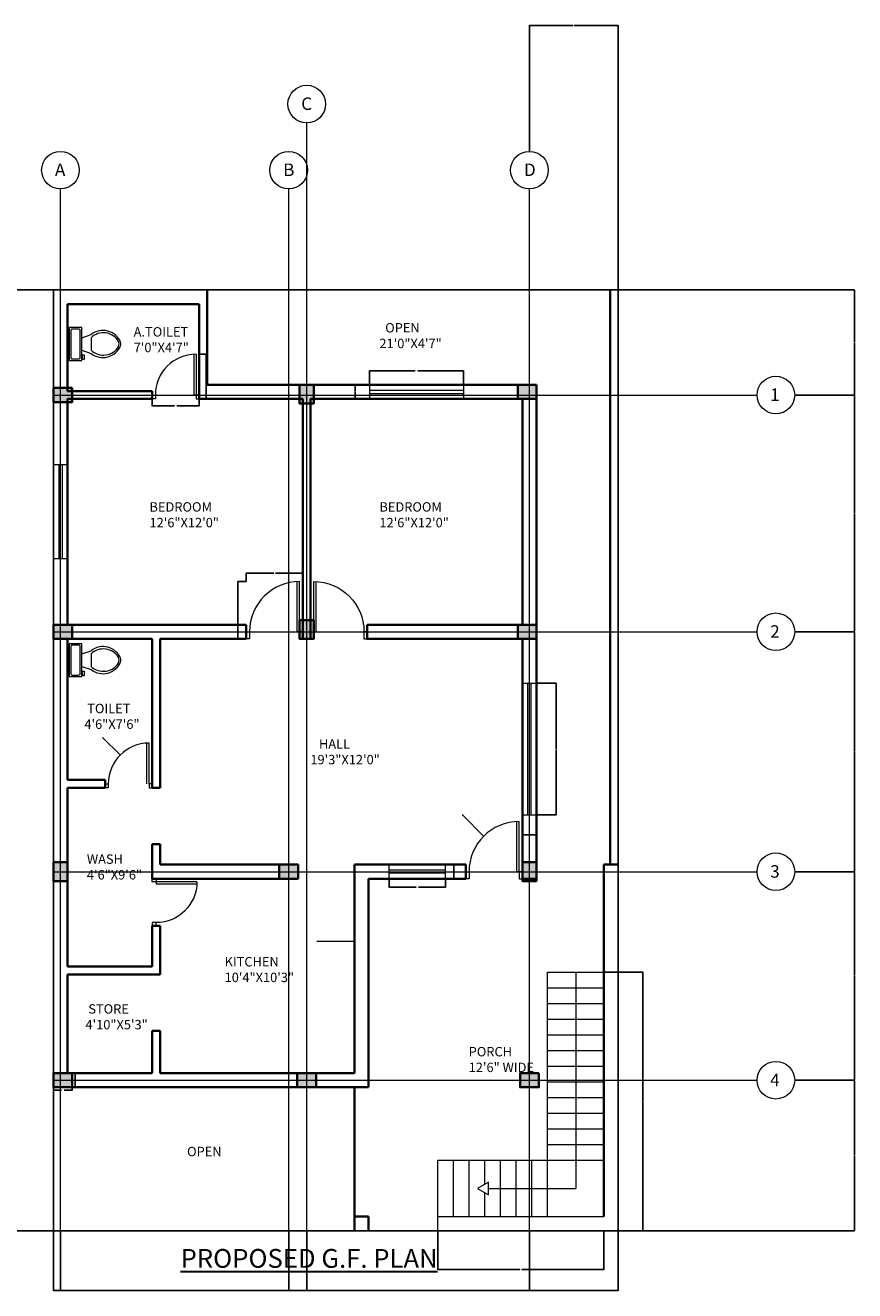
# Model space of a CAD drawing. Units: inches. Extents: x 1602 to 2642, y 1463 to 2270.
# Tile 5 of 5: x 2113 to 2642, y 1463 to 2270. Entities that reach past the tile are written whole.
import ezdxf

# ---------------------------------------------------------------- set-up
doc = ezdxf.new("R2010")
doc.units = ezdxf.units.IN
for name, color, linetype, lineweight in [('A-ANNO-DIMS', 2, 'Continuous', 18), ('A-ANNO-TEXT', 7, 'Continuous', 30), ('A-AREA-IDEN', 7, 'Continuous', 18), ('A-COLS', 7, 'Continuous', 35), ('A-DOOR', 3, 'Continuous', 18), ('A-FLOR-CASE', 9, 'Continuous', 18), ('A-FLOR-FIXT', 8, 'Continuous', 18), ('A-FLOR-STRS', 7, 'Continuous', 18), ('A-GLAZ', 4, 'Continuous', 18), ('A-GRID', 8, 'Continuous', 13), ('A-WALL', 7, 'Continuous', 35), ('C-PROP', 7, 'Continuous', 25)]:
    doc.layers.add(name, color=color, linetype=linetype, lineweight=lineweight)
doc.styles.get("Standard").update_dxf_attribs({"font": 'arial.ttf'})
doc.dimstyles.get("Standard").update_dxf_attribs({"dimtxt": 0.18, "dimasz": 0.18, "dimexe": 0.18, "dimexo": 0.0625, "dimgap": 0.09, "dimtad": 0, "dimtih": 1, "dimtoh": 1, "dimdec": 4, "dimzin": 0, "dimdsep": 46, "dimtxsty": 'Standard', "dimcen": 0.09, "dimadec": 0, "dimazin": 0, "dimtfac": 1, "dimtdec": 4, "dimtofl": 0, "dimtmove": 0, "dimatfit": 3, "dimfxl": 1, "dimtolj": 1, "dimtzin": 0, "dimarcsym": 0})

# ---------------------------------------------------------------- blocks, each defined once
blk = doc.blocks.new('*U3')
for p, q in [((-8, -8.5), (-8, -8)), ((-7, -8), (-7, -9.5)), ((-4, -8), (-6, -14)), ((4, -8), (6, -14)), ((9.5, -6), (9.5, -2)), ((-10, -8.5), (-8, -8.5)), ((-10, -9.5), (-10, -8.5)), ((-7, -9.5), (-10, -9.5)), ((4, -14), (-4, -14))]:
    blk.add_line(p, q)
blk.add_lwpolyline([(10.5, -8), (10.5, 0), (-10.5, 0), (-10.5, -8)], close=True)
for points in [[(-9.5, -2), (-9.5, -6)], [(8.5, -1), (-8.5, -1)], [(-8.5, -7), (8.5, -7)]]:
    blk.add_lwpolyline(points)
for centre, radius, start, end in [((-8.62, -1.88), 0.884, 81.8699, 188.1301), ((-8.62, -6.12), 0.884, 171.8699, 278.1301), ((8.62, -1.88), 0.884, 351.8699, 98.1301), ((8.62, -6.12), 0.884, 261.8699, 8.1301), ((3.52, -21.58), 12.17, 141.46911, 247.97143), ((4.2, -21.82), 11.33, 136.36773, 238.94682), ((-3.52, -21.58), 12.17, 292.02843, 38.53071), ((-4.2, -21.82), 11.33, 301.05301, 43.63209), ((0, -27.88), 4, 245.73182, 294.26817), ((0, -29), 4, 254.86053, 285.13947)]:
    blk.add_arc(centre, radius, start, end)
blk = doc.blocks.new('DOOR-SWING-26IN')
for p, q in [((26.5, 28.46), (26.5, 2.5)), ((28, 28.5), (28, 2.5)), ((0, 2.5), (2, 2.5)), ((2, 2.5), (2, 0)), ((28, 2.5), (26.5, 2.5)), ((30, 2.5), (28, 2.5)), ((28, 2.5), (28, 0)), ((2, 0), (0, 0)), ((28, 0), (30, 0))]:
    blk.add_line(p, q)
blk.add_arc((28, 2.5), 26, 90, 180)
blk = doc.blocks.new('DOOR-SWING-32IN')
for p, q in [((32.5, 4.5), (32.5, 36.46)), ((34, 4.5), (34, 36.5)), ((0, 4.5), (2, 4.5)), ((2, 0), (0, 0)), ((2, 4.5), (2, 0)), ((34, 4.5), (32.5, 4.5)), ((36, 4.5), (34, 4.5)), ((34, 4.5), (34, 0)), ((34, 0), (36, 0))]:
    blk.add_line(p, q)
blk.add_arc((34, 4.5), 32, 90, 180)
blk = doc.blocks.new('WIN-60IN')
for p, q in [((0, 0), (0, 9)), ((60, 0), (60, 9)), ((60, 5.5), (0, 5.5)), ((60, 3.5), (0, 3.5))]:
    blk.add_line(p, q)
blk = doc.blocks.new('WIN-36IN')
for p, q in [((0, 0), (0, 9)), ((36, 0), (36, 9)), ((36, 5.5), (0, 5.5)), ((36, 3.5), (0, 3.5))]:
    blk.add_line(p, q)
blk = doc.blocks.new('WIN-84IN')
for p, q in [((0, 84), (9, 84)), ((3.5, 0), (3.5, 84)), ((5.5, 0), (5.5, 84)), ((0, 0), (9, 0))]:
    blk.add_line(p, q)
blk = doc.blocks.new('COL-12X9')
h = blk.add_hatch(color=256)
h.dxf.hatch_style = 1
h.paths.add_polyline_path([(12, 0), (12, 9), (0, 9), (0, 0)])
blk.add_lwpolyline([(12, 9), (12, 0), (0, 0), (0, 9)], close=True)
blk = doc.blocks.new('STAIR-PORCH-RETURN')
for p, q in [((70, 9), (70, 165)), ((70, 165), (106, 165)), ((88, 165), (88, 27)), ((70, 155), (106, 155)), ((70, 145), (106, 145)), ((70, 135), (106, 135)), ((70, 125), (106, 125)), ((70, 115), (106, 115)), ((70, 105), (106, 105)), ((70, 95), (106, 95)), ((70, 85), (106, 85)), ((70, 75), (106, 75)), ((70, 65), (106, 65)), ((70, 55), (106, 55)), ((0, 45), (106, 45)), ((0, 0), (0, 45)), ((10, 9), (10, 45)), ((20, 9), (20, 45)), ((30, 29.72), (30, 45)), ((40, 9), (40, 45)), ((50, 9), (50, 45)), ((60, 9), (60, 45)), ((30, 9), (30, 24.28)), ((32.36, 27), (88, 27)), ((0, 9), (106, 9))]:
    blk.add_line(p, q)
blk.add_lwpolyline([(25.29, 27), (32.36, 22.92), (32.36, 31.08)], close=True)
blk = doc.blocks.new('*D25')
at = {"layer": 'A-ANNO-DIMS', "color": 0, "lineweight": -2, "transparency": 16777216}
for p, q in [((2130.66, 1592.19), (2130.66, 1590.27)), ((2130.84, 1590.45), (2135.8, 1590.45)), ((2142.48, 1590.45), (2137.51, 1590.45)), ((2142.66, 1592.19), (2142.66, 1590.27))]:
    blk.add_line(p, q, dxfattribs=at)
at = {"layer": 'A-ANNO-DIMS', "color": 0, "transparency": 16777216}
for points in [[(2130.84, 1590.48), (2130.84, 1590.42), (2130.66, 1590.45)], [(2142.48, 1590.48), (2142.48, 1590.42), (2142.66, 1590.45)]]:
    blk.add_solid(points, dxfattribs=at)
at = {"layer": 'Defpoints', "color": 0, "transparency": 16777216}
for p in [(2130.66, 1592.25), (2142.66, 1592.25), (2142.66, 1590.45)]:
    blk.add_point(p, dxfattribs=at)
at = {"layer": 'A-ANNO-DIMS', "color": 0, "transparency": 16777216, "insert": (2136.66, 1590.45), "char_height": 0.18, "attachment_point": 5}
blk.add_mtext('\\A1;COL. 12 TYP.', dxfattribs=at)
blk = doc.blocks.new('*D26')
at = {"layer": 'A-ANNO-DIMS', "color": 0, "lineweight": -2, "transparency": 16777216}
for p, q in [((2142.72, 1601.25), (2144.64, 1601.25)), ((2144.46, 1601.07), (2144.46, 1596.93)), ((2142.72, 1592.25), (2144.64, 1592.25)), ((2144.46, 1592.43), (2144.46, 1596.57))]:
    blk.add_line(p, q, dxfattribs=at)
at = {"layer": 'A-ANNO-DIMS', "color": 0, "transparency": 16777216}
for points in [[(2144.43, 1601.07), (2144.49, 1601.07), (2144.46, 1601.25)], [(2144.43, 1592.43), (2144.49, 1592.43), (2144.46, 1592.25)]]:
    blk.add_solid(points, dxfattribs=at)
at = {"layer": 'Defpoints', "color": 0, "transparency": 16777216}
for p in [(2142.66, 1601.25), (2144.46, 1601.25), (2142.66, 1592.25)]:
    blk.add_point(p, dxfattribs=at)
at = {"layer": 'A-ANNO-DIMS', "color": 0, "transparency": 16777216, "insert": (2144.46, 1596.75), "char_height": 0.18, "attachment_point": 5}
blk.add_mtext('\\A1;9 TYP.', dxfattribs=at)
blk = doc.blocks.new('*D27')
at = {"layer": 'A-ANNO-DIMS', "color": 0, "lineweight": -2, "transparency": 16777216}
for p, q in [((2253.59, 1914.75), (2248, 1914.75)), ((2248.18, 1914.57), (2248.18, 1896.68)), ((2248.18, 1878.43), (2248.18, 1896.32)), ((2253.59, 1878.25), (2248, 1878.25))]:
    blk.add_line(p, q, dxfattribs=at)
at = {"layer": 'A-ANNO-DIMS', "color": 0, "transparency": 16777216}
for points in [[(2248.15, 1914.57), (2248.21, 1914.57), (2248.18, 1914.75)], [(2248.15, 1878.43), (2248.21, 1878.43), (2248.18, 1878.25)]]:
    blk.add_solid(points, dxfattribs=at)
at = {"layer": 'Defpoints', "color": 0, "transparency": 16777216}
for p in [(2248.18, 1914.75), (2253.66, 1914.75), (2253.66, 1878.25)]:
    blk.add_point(p, dxfattribs=at)
at = {"layer": 'A-ANNO-DIMS', "color": 0, "transparency": 16777216, "insert": (2248.18, 1896.5), "char_height": 0.18, "attachment_point": 5}
blk.add_mtext('\\A1;D1 37 TYP.', dxfattribs=at)
blk = doc.blocks.new('*D28')
at = {"layer": 'A-ANNO-DIMS', "color": 0, "lineweight": -2, "transparency": 16777216}
for p, q in [((2253.66, 1914.81), (2253.66, 1920.4)), ((2253.84, 1920.22), (2271.13, 1920.22)), ((2289.48, 1920.22), (2272.18, 1920.22)), ((2289.66, 1914.81), (2289.66, 1920.4))]:
    blk.add_line(p, q, dxfattribs=at)
at = {"layer": 'A-ANNO-DIMS', "color": 0, "transparency": 16777216}
for points in [[(2253.84, 1920.25), (2253.84, 1920.19), (2253.66, 1920.22)], [(2289.48, 1920.25), (2289.48, 1920.19), (2289.66, 1920.22)]]:
    blk.add_solid(points, dxfattribs=at)
at = {"layer": 'Defpoints', "color": 0, "transparency": 16777216}
for p in [(2253.66, 1914.75), (2289.66, 1920.22), (2289.66, 1914.75)]:
    blk.add_point(p, dxfattribs=at)
at = {"layer": 'A-ANNO-DIMS', "color": 0, "transparency": 16777216, "insert": (2271.66, 1920.22), "char_height": 0.18, "attachment_point": 5}
blk.add_mtext('\\A1;36 TYP.', dxfattribs=at)
blk = doc.blocks.new('*D29')
at = {"layer": 'A-ANNO-DIMS', "color": 0, "lineweight": -2, "transparency": 16777216}
for p, q in [((2193.66, 2031.19), (2193.66, 2026.57)), ((2193.84, 2026.75), (2207.94, 2026.75)), ((2223.48, 2026.75), (2209.38, 2026.75)), ((2223.66, 2031.19), (2223.66, 2026.57))]:
    blk.add_line(p, q, dxfattribs=at)
at = {"layer": 'A-ANNO-DIMS', "color": 0, "transparency": 16777216}
for points in [[(2193.84, 2026.78), (2193.84, 2026.72), (2193.66, 2026.75)], [(2223.48, 2026.78), (2223.48, 2026.72), (2223.66, 2026.75)]]:
    blk.add_solid(points, dxfattribs=at)
at = {"layer": 'Defpoints', "color": 0, "transparency": 16777216}
for p in [(2193.66, 2031.25), (2223.66, 2031.25), (2223.66, 2026.75)]:
    blk.add_point(p, dxfattribs=at)
at = {"layer": 'A-ANNO-DIMS', "color": 0, "transparency": 16777216, "insert": (2208.66, 2026.75), "char_height": 0.18, "attachment_point": 5}
blk.add_mtext('\\A1;D2 30 TYP.', dxfattribs=at)
blk = doc.blocks.new('*D30')
at = {"layer": 'A-ANNO-DIMS', "color": 0, "lineweight": -2, "transparency": 16777216}
for p, q in [((2223.72, 2059.75), (2228.34, 2059.75)), ((2228.16, 2059.57), (2228.16, 2045.68)), ((2228.16, 2031.43), (2228.16, 2045.32)), ((2223.72, 2031.25), (2228.34, 2031.25))]:
    blk.add_line(p, q, dxfattribs=at)
at = {"layer": 'A-ANNO-DIMS', "color": 0, "transparency": 16777216}
for points in [[(2228.13, 2059.57), (2228.19, 2059.57), (2228.16, 2059.75)], [(2228.13, 2031.43), (2228.19, 2031.43), (2228.16, 2031.25)]]:
    blk.add_solid(points, dxfattribs=at)
at = {"layer": 'Defpoints', "color": 0, "transparency": 16777216}
for p in [(2223.66, 2059.75), (2228.16, 2059.75), (2223.66, 2031.25)]:
    blk.add_point(p, dxfattribs=at)
at = {"layer": 'A-ANNO-DIMS', "color": 0, "transparency": 16777216, "insert": (2228.16, 2045.5), "char_height": 0.18, "attachment_point": 5}
blk.add_mtext('\\A1;29 TYP.', dxfattribs=at)
blk = doc.blocks.new('*D31')
at = {"layer": 'A-ANNO-DIMS', "color": 0, "lineweight": -2, "transparency": 16777216}
for p, q in [((2332.16, 2040.31), (2332.16, 2049.43)), ((2332.34, 2049.25), (2361.4, 2049.25)), ((2391.98, 2049.25), (2362.91, 2049.25)), ((2392.16, 2040.31), (2392.16, 2049.43))]:
    blk.add_line(p, q, dxfattribs=at)
at = {"layer": 'A-ANNO-DIMS', "color": 0, "transparency": 16777216}
for points in [[(2332.34, 2049.28), (2332.34, 2049.22), (2332.16, 2049.25)], [(2391.98, 2049.28), (2391.98, 2049.22), (2392.16, 2049.25)]]:
    blk.add_solid(points, dxfattribs=at)
at = {"layer": 'Defpoints', "color": 0, "transparency": 16777216}
for p in [(2332.16, 2049.25), (2332.16, 2040.25), (2392.16, 2040.25)]:
    blk.add_point(p, dxfattribs=at)
at = {"layer": 'A-ANNO-DIMS', "color": 0, "transparency": 16777216, "insert": (2362.16, 2049.25), "char_height": 0.18, "attachment_point": 5}
blk.add_mtext('\\A1;W1 60 TYP.', dxfattribs=at)
blk = doc.blocks.new('*D32')
at = {"layer": 'A-ANNO-DIMS', "color": 0, "lineweight": -2, "transparency": 16777216}
for p, q in [((2332.09, 2040.25), (2322.98, 2040.25)), ((2323.16, 2040.07), (2323.16, 2035.93)), ((2323.16, 2031.43), (2323.16, 2035.57)), ((2332.09, 2031.25), (2322.98, 2031.25))]:
    blk.add_line(p, q, dxfattribs=at)
at = {"layer": 'A-ANNO-DIMS', "color": 0, "transparency": 16777216}
for points in [[(2323.13, 2040.07), (2323.19, 2040.07), (2323.16, 2040.25)], [(2323.13, 2031.43), (2323.19, 2031.43), (2323.16, 2031.25)]]:
    blk.add_solid(points, dxfattribs=at)
at = {"layer": 'Defpoints', "color": 0, "transparency": 16777216}
for p in [(2332.16, 2040.25), (2323.16, 2031.25), (2332.16, 2031.25)]:
    blk.add_point(p, dxfattribs=at)
at = {"layer": 'A-ANNO-DIMS', "color": 0, "transparency": 16777216, "insert": (2323.16, 2035.75), "char_height": 0.18, "attachment_point": 5}
blk.add_mtext('\\A1;9 TYP.', dxfattribs=at)
blk = doc.blocks.new('*D33')
at = {"layer": 'A-ANNO-DIMS', "color": 0, "lineweight": -2, "transparency": 16777216}
for p, q in [((2344.66, 1725.19), (2344.66, 1719.67)), ((2344.84, 1719.85), (2361.9, 1719.85)), ((2380.48, 1719.85), (2363.41, 1719.85)), ((2380.66, 1725.19), (2380.66, 1719.67))]:
    blk.add_line(p, q, dxfattribs=at)
at = {"layer": 'A-ANNO-DIMS', "color": 0, "transparency": 16777216}
for points in [[(2344.84, 1719.88), (2344.84, 1719.82), (2344.66, 1719.85)], [(2380.48, 1719.88), (2380.48, 1719.82), (2380.66, 1719.85)]]:
    blk.add_solid(points, dxfattribs=at)
at = {"layer": 'Defpoints', "color": 0, "transparency": 16777216}
for p in [(2344.66, 1725.25), (2380.66, 1725.25), (2380.66, 1719.85)]:
    blk.add_point(p, dxfattribs=at)
at = {"layer": 'A-ANNO-DIMS', "color": 0, "transparency": 16777216, "insert": (2362.66, 1719.85), "char_height": 0.18, "attachment_point": 5}
blk.add_mtext('\\A1;W2 36 TYP.', dxfattribs=at)
blk = doc.blocks.new('*D34')
at = {"layer": 'A-ANNO-DIMS', "color": 0, "lineweight": -2, "transparency": 16777216}
for p, q in [((2380.72, 1734.25), (2386.24, 1734.25)), ((2386.06, 1734.07), (2386.06, 1729.93)), ((2386.06, 1725.43), (2386.06, 1729.57)), ((2380.72, 1725.25), (2386.24, 1725.25))]:
    blk.add_line(p, q, dxfattribs=at)
at = {"layer": 'A-ANNO-DIMS', "color": 0, "transparency": 16777216}
for points in [[(2386.03, 1734.07), (2386.09, 1734.07), (2386.06, 1734.25)], [(2386.03, 1725.43), (2386.09, 1725.43), (2386.06, 1725.25)]]:
    blk.add_solid(points, dxfattribs=at)
at = {"layer": 'Defpoints', "color": 0, "transparency": 16777216}
for p in [(2380.66, 1734.25), (2386.06, 1734.25), (2380.66, 1725.25)]:
    blk.add_point(p, dxfattribs=at)
at = {"layer": 'A-ANNO-DIMS', "color": 0, "transparency": 16777216, "insert": (2386.06, 1729.75), "char_height": 0.18, "attachment_point": 5}
blk.add_mtext('\\A1;9 TYP.', dxfattribs=at)
blk = doc.blocks.new('*D35')
at = {"layer": 'A-ANNO-DIMS', "color": 0, "lineweight": -2, "transparency": 16777216}
for p, q in [((2438.72, 1849.94), (2451.44, 1849.94)), ((2451.26, 1849.76), (2451.26, 1808.12)), ((2451.26, 1766.12), (2451.26, 1807.76)), ((2438.72, 1765.94), (2451.44, 1765.94))]:
    blk.add_line(p, q, dxfattribs=at)
at = {"layer": 'A-ANNO-DIMS', "color": 0, "transparency": 16777216}
for points in [[(2451.23, 1849.76), (2451.29, 1849.76), (2451.26, 1849.94)], [(2451.23, 1766.12), (2451.29, 1766.12), (2451.26, 1765.94)]]:
    blk.add_solid(points, dxfattribs=at)
at = {"layer": 'Defpoints', "color": 0, "transparency": 16777216}
for p in [(2438.66, 1849.94), (2451.26, 1849.94), (2438.66, 1765.94)]:
    blk.add_point(p, dxfattribs=at)
at = {"layer": 'A-ANNO-DIMS', "color": 0, "transparency": 16777216, "insert": (2451.26, 1807.94), "char_height": 0.18, "attachment_point": 5}
blk.add_mtext('\\A1;W3 84 TYP.', dxfattribs=at)
blk = doc.blocks.new('*D36')
at = {"layer": 'A-ANNO-DIMS', "color": 0, "lineweight": -2, "transparency": 16777216}
for p, q in [((2429.66, 1765.88), (2429.66, 1753.16)), ((2438.66, 1765.88), (2438.66, 1753.16)), ((2429.84, 1753.34), (2433.7, 1753.34)), ((2438.48, 1753.34), (2434.61, 1753.34))]:
    blk.add_line(p, q, dxfattribs=at)
at = {"layer": 'A-ANNO-DIMS', "color": 0, "transparency": 16777216}
for points in [[(2429.84, 1753.37), (2429.84, 1753.31), (2429.66, 1753.34)], [(2438.48, 1753.37), (2438.48, 1753.31), (2438.66, 1753.34)]]:
    blk.add_solid(points, dxfattribs=at)
at = {"layer": 'Defpoints', "color": 0, "transparency": 16777216}
for p in [(2429.66, 1765.94), (2438.66, 1765.94), (2438.66, 1753.34)]:
    blk.add_point(p, dxfattribs=at)
at = {"layer": 'A-ANNO-DIMS', "color": 0, "transparency": 16777216, "insert": (2434.16, 1753.34), "char_height": 0.18, "attachment_point": 5}
blk.add_mtext('\\A1;9 TYP.', dxfattribs=at)
blk = doc.blocks.new('*D37')
at = {"layer": 'A-ANNO-DIMS', "color": 0, "lineweight": -2, "transparency": 16777216}
for p, q in [((2481.72, 1665.75), (2506.59, 1665.75)), ((2506.41, 1665.57), (2506.41, 1583.43)), ((2506.41, 1500.93), (2506.41, 1583.06)), ((2481.72, 1500.75), (2506.59, 1500.75))]:
    blk.add_line(p, q, dxfattribs=at)
at = {"layer": 'A-ANNO-DIMS', "color": 0, "transparency": 16777216}
for points in [[(2506.38, 1665.57), (2506.44, 1665.57), (2506.41, 1665.75)], [(2506.38, 1500.93), (2506.44, 1500.93), (2506.41, 1500.75)]]:
    blk.add_solid(points, dxfattribs=at)
at = {"layer": 'Defpoints', "color": 0, "transparency": 16777216}
for p in [(2481.66, 1665.75), (2506.41, 1665.75), (2481.66, 1500.75)]:
    blk.add_point(p, dxfattribs=at)
at = {"layer": 'A-ANNO-DIMS', "color": 0, "transparency": 16777216, "insert": (2506.41, 1583.25), "char_height": 0.18, "attachment_point": 5}
blk.add_mtext('\\A1;PORCH STAIR 165 TYP.', dxfattribs=at)
blk = doc.blocks.new('*D38')
at = {"layer": 'A-ANNO-DIMS', "color": 0, "lineweight": -2, "transparency": 16777216}
for p, q in [((2375.66, 1500.69), (2375.66, 1475.82)), ((2481.66, 1500.69), (2481.66, 1475.82)), ((2375.84, 1476), (2428.07, 1476)), ((2481.48, 1476), (2429.25, 1476))]:
    blk.add_line(p, q, dxfattribs=at)
at = {"layer": 'A-ANNO-DIMS', "color": 0, "transparency": 16777216}
for points in [[(2375.84, 1476.03), (2375.84, 1475.97), (2375.66, 1476)], [(2481.48, 1476.03), (2481.48, 1475.97), (2481.66, 1476)]]:
    blk.add_solid(points, dxfattribs=at)
at = {"layer": 'Defpoints', "color": 0, "transparency": 16777216}
for p in [(2375.66, 1500.75), (2481.66, 1500.75), (2481.66, 1476)]:
    blk.add_point(p, dxfattribs=at)
at = {"layer": 'A-ANNO-DIMS', "color": 0, "transparency": 16777216, "insert": (2428.66, 1476), "char_height": 0.18, "attachment_point": 5}
blk.add_mtext('\\A1;106 TYP.', dxfattribs=at)
blk = doc.blocks.new('*D41')
at = {"layer": 'A-ANNO-DIMS', "color": 0, "lineweight": -2, "transparency": 16777216}
for p, q in [((2130.66, 1500.69), (2130.66, 1462.52)), ((2490.66, 1500.69), (2490.66, 1462.52)), ((2130.84, 1462.7), (2310.37, 1462.7)), ((2490.48, 1462.7), (2310.94, 1462.7))]:
    blk.add_line(p, q, dxfattribs=at)
at = {"layer": 'A-ANNO-DIMS', "color": 0, "transparency": 16777216}
for points in [[(2130.84, 1462.73), (2130.84, 1462.67), (2130.66, 1462.7)], [(2490.48, 1462.73), (2490.48, 1462.67), (2490.66, 1462.7)]]:
    blk.add_solid(points, dxfattribs=at)
at = {"layer": 'Defpoints', "color": 0, "transparency": 16777216}
for p in [(2130.66, 1500.75), (2490.66, 1500.75), (2490.66, 1462.7)]:
    blk.add_point(p, dxfattribs=at)
at = {"layer": 'A-ANNO-DIMS', "color": 0, "transparency": 16777216, "insert": (2310.66, 1462.7), "char_height": 0.18, "attachment_point": 5}
blk.add_mtext('\\A1;360', dxfattribs=at)
blk = doc.blocks.new('*D42')
at = {"layer": 'A-ANNO-DIMS', "color": 0, "lineweight": -2, "transparency": 16777216}
for p, q in [((2130.59, 2100.75), (2042.46, 2100.75)), ((2042.64, 2100.57), (2042.64, 1800.93)), ((2042.64, 1500.93), (2042.64, 1800.57)), ((2130.59, 1500.75), (2042.46, 1500.75))]:
    blk.add_line(p, q, dxfattribs=at)
at = {"layer": 'A-ANNO-DIMS', "color": 0, "transparency": 16777216}
for points in [[(2042.61, 2100.57), (2042.67, 2100.57), (2042.64, 2100.75)], [(2042.61, 1500.93), (2042.67, 1500.93), (2042.64, 1500.75)]]:
    blk.add_solid(points, dxfattribs=at)
at = {"layer": 'Defpoints', "color": 0, "transparency": 16777216}
for p in [(2042.64, 2100.75), (2130.66, 2100.75), (2130.66, 1500.75)]:
    blk.add_point(p, dxfattribs=at)
at = {"layer": 'A-ANNO-DIMS', "color": 0, "transparency": 16777216, "insert": (2042.64, 1800.75), "char_height": 0.18, "attachment_point": 5}
blk.add_mtext('\\A1;600', dxfattribs=at)
blk = doc.blocks.new('*D43')
at = {"layer": 'A-ANNO-DIMS', "color": 0, "lineweight": -2, "transparency": 16777216}
for p, q in [((2135.16, 1500.69), (2135.16, 1462.52)), ((2280.66, 1500.69), (2280.66, 1462.52)), ((2135.34, 1462.7), (2207.52, 1462.7)), ((2280.48, 1462.7), (2208.29, 1462.7))]:
    blk.add_line(p, q, dxfattribs=at)
at = {"layer": 'A-ANNO-DIMS', "color": 0, "transparency": 16777216}
for points in [[(2135.34, 1462.73), (2135.34, 1462.67), (2135.16, 1462.7)], [(2280.48, 1462.73), (2280.48, 1462.67), (2280.66, 1462.7)]]:
    blk.add_solid(points, dxfattribs=at)
at = {"layer": 'Defpoints', "color": 0, "transparency": 16777216}
for p in [(2135.16, 1500.75), (2280.66, 1500.75), (2280.66, 1462.7)]:
    blk.add_point(p, dxfattribs=at)
at = {"layer": 'A-ANNO-DIMS', "color": 0, "transparency": 16777216, "insert": (2207.91, 1462.7), "char_height": 0.18, "attachment_point": 5}
blk.add_mtext('\\A1;145.5', dxfattribs=at)
blk = doc.blocks.new('*D44')
at = {"layer": 'A-ANNO-DIMS', "color": 0, "lineweight": -2, "transparency": 16777216}
for p, q in [((2280.66, 1500.69), (2280.66, 1462.52)), ((2292.16, 1500.69), (2292.16, 1462.52)), ((2280.84, 1462.7), (2286.09, 1462.7)), ((2291.98, 1462.7), (2286.72, 1462.7))]:
    blk.add_line(p, q, dxfattribs=at)
at = {"layer": 'A-ANNO-DIMS', "color": 0, "transparency": 16777216}
for points in [[(2280.84, 1462.73), (2280.84, 1462.67), (2280.66, 1462.7)], [(2291.98, 1462.73), (2291.98, 1462.67), (2292.16, 1462.7)]]:
    blk.add_solid(points, dxfattribs=at)
at = {"layer": 'Defpoints', "color": 0, "transparency": 16777216}
for p in [(2280.66, 1500.75), (2292.16, 1500.75), (2292.16, 1462.7)]:
    blk.add_point(p, dxfattribs=at)
at = {"layer": 'A-ANNO-DIMS', "color": 0, "transparency": 16777216, "insert": (2286.41, 1462.7), "char_height": 0.18, "attachment_point": 5}
blk.add_mtext('\\A1;11.5', dxfattribs=at)
blk = doc.blocks.new('*D45')
at = {"layer": 'A-ANNO-DIMS', "color": 0, "lineweight": -2, "transparency": 16777216}
for p, q in [((2292.16, 1500.69), (2292.16, 1462.52)), ((2434.16, 1500.69), (2434.16, 1462.52)), ((2292.34, 1462.7), (2362.88, 1462.7)), ((2433.98, 1462.7), (2363.44, 1462.7))]:
    blk.add_line(p, q, dxfattribs=at)
at = {"layer": 'A-ANNO-DIMS', "color": 0, "transparency": 16777216}
for points in [[(2292.34, 1462.73), (2292.34, 1462.67), (2292.16, 1462.7)], [(2433.98, 1462.73), (2433.98, 1462.67), (2434.16, 1462.7)]]:
    blk.add_solid(points, dxfattribs=at)
at = {"layer": 'Defpoints', "color": 0, "transparency": 16777216}
for p in [(2292.16, 1500.75), (2434.16, 1500.75), (2434.16, 1462.7)]:
    blk.add_point(p, dxfattribs=at)
at = {"layer": 'A-ANNO-DIMS', "color": 0, "transparency": 16777216, "insert": (2363.16, 1462.7), "char_height": 0.18, "attachment_point": 5}
blk.add_mtext('\\A1;142', dxfattribs=at)
blk = doc.blocks.new('*D46')
at = {"layer": 'A-ANNO-DIMS', "color": 0, "lineweight": -2, "transparency": 16777216}
for p, q in [((2434.16, 2189.21), (2434.16, 2269.53)), ((2434.34, 2269.35), (2462.08, 2269.35)), ((2490.48, 2269.35), (2462.73, 2269.35)), ((2490.66, 2100.81), (2490.66, 2269.53))]:
    blk.add_line(p, q, dxfattribs=at)
at = {"layer": 'A-ANNO-DIMS', "color": 0, "transparency": 16777216}
for points in [[(2434.34, 2269.38), (2434.34, 2269.32), (2434.16, 2269.35)], [(2490.48, 2269.38), (2490.48, 2269.32), (2490.66, 2269.35)]]:
    blk.add_solid(points, dxfattribs=at)
at = {"layer": 'Defpoints', "color": 0, "transparency": 16777216}
for p in [(2490.66, 2269.35), (2434.16, 2189.15), (2490.66, 2100.75)]:
    blk.add_point(p, dxfattribs=at)
at = {"layer": 'A-ANNO-DIMS', "color": 0, "transparency": 16777216, "insert": (2462.41, 2269.35), "char_height": 0.18, "attachment_point": 5}
blk.add_mtext('\\A1;56.5', dxfattribs=at)
blk = doc.blocks.new('*D47')
at = {"layer": 'A-ANNO-DIMS', "color": 0, "lineweight": -2, "transparency": 16777216}
for p, q in [((2603.33, 1596.75), (2641.5, 1596.75)), ((2641.32, 1596.57), (2641.32, 1548.93)), ((2641.32, 1500.93), (2641.32, 1548.57)), ((2490.72, 1500.75), (2641.5, 1500.75))]:
    blk.add_line(p, q, dxfattribs=at)
at = {"layer": 'A-ANNO-DIMS', "color": 0, "transparency": 16777216}
for points in [[(2641.29, 1596.57), (2641.35, 1596.57), (2641.32, 1596.75)], [(2641.29, 1500.93), (2641.35, 1500.93), (2641.32, 1500.75)]]:
    blk.add_solid(points, dxfattribs=at)
at = {"layer": 'Defpoints', "color": 0, "transparency": 16777216}
for p in [(2603.27, 1596.75), (2641.32, 1596.75), (2490.66, 1500.75)]:
    blk.add_point(p, dxfattribs=at)
at = {"layer": 'A-ANNO-DIMS', "color": 0, "transparency": 16777216, "insert": (2641.32, 1548.75), "char_height": 0.18, "attachment_point": 5}
blk.add_mtext('\\A1;96', dxfattribs=at)
blk = doc.blocks.new('*D48')
at = {"layer": 'A-ANNO-DIMS', "color": 0, "lineweight": -2, "transparency": 16777216}
for p, q in [((2603.33, 1729.75), (2641.5, 1729.75)), ((2641.32, 1729.57), (2641.32, 1663.43)), ((2641.32, 1596.93), (2641.32, 1663.07)), ((2603.33, 1596.75), (2641.5, 1596.75))]:
    blk.add_line(p, q, dxfattribs=at)
at = {"layer": 'A-ANNO-DIMS', "color": 0, "transparency": 16777216}
for points in [[(2641.29, 1729.57), (2641.35, 1729.57), (2641.32, 1729.75)], [(2641.29, 1596.93), (2641.35, 1596.93), (2641.32, 1596.75)]]:
    blk.add_solid(points, dxfattribs=at)
at = {"layer": 'Defpoints', "color": 0, "transparency": 16777216}
for p in [(2603.27, 1729.75), (2641.32, 1729.75), (2603.27, 1596.75)]:
    blk.add_point(p, dxfattribs=at)
at = {"layer": 'A-ANNO-DIMS', "color": 0, "transparency": 16777216, "insert": (2641.32, 1663.25), "char_height": 0.18, "attachment_point": 5}
blk.add_mtext('\\A1;133', dxfattribs=at)
blk = doc.blocks.new('*D49')
at = {"layer": 'A-ANNO-DIMS', "color": 0, "lineweight": -2, "transparency": 16777216}
for p, q in [((2603.33, 1882.75), (2641.5, 1882.75)), ((2641.32, 1882.57), (2641.32, 1806.43)), ((2641.32, 1729.93), (2641.32, 1806.07)), ((2603.33, 1729.75), (2641.5, 1729.75))]:
    blk.add_line(p, q, dxfattribs=at)
at = {"layer": 'A-ANNO-DIMS', "color": 0, "transparency": 16777216}
for points in [[(2641.29, 1882.57), (2641.35, 1882.57), (2641.32, 1882.75)], [(2641.29, 1729.93), (2641.35, 1729.93), (2641.32, 1729.75)]]:
    blk.add_solid(points, dxfattribs=at)
at = {"layer": 'Defpoints', "color": 0, "transparency": 16777216}
for p in [(2603.27, 1882.75), (2641.32, 1882.75), (2603.27, 1729.75)]:
    blk.add_point(p, dxfattribs=at)
at = {"layer": 'A-ANNO-DIMS', "color": 0, "transparency": 16777216, "insert": (2641.32, 1806.25), "char_height": 0.18, "attachment_point": 5}
blk.add_mtext('\\A1;153', dxfattribs=at)
blk = doc.blocks.new('*D50')
at = {"layer": 'A-ANNO-DIMS', "color": 0, "lineweight": -2, "transparency": 16777216}
for p, q in [((2603.33, 2033.75), (2641.5, 2033.75)), ((2641.32, 2033.57), (2641.32, 1958.43)), ((2641.32, 1882.93), (2641.32, 1958.07)), ((2603.33, 1882.75), (2641.5, 1882.75))]:
    blk.add_line(p, q, dxfattribs=at)
at = {"layer": 'A-ANNO-DIMS', "color": 0, "transparency": 16777216}
for points in [[(2641.29, 2033.57), (2641.35, 2033.57), (2641.32, 2033.75)], [(2641.29, 1882.93), (2641.35, 1882.93), (2641.32, 1882.75)]]:
    blk.add_solid(points, dxfattribs=at)
at = {"layer": 'Defpoints', "color": 0, "transparency": 16777216}
for p in [(2603.27, 2033.75), (2641.32, 2033.75), (2603.27, 1882.75)]:
    blk.add_point(p, dxfattribs=at)
at = {"layer": 'A-ANNO-DIMS', "color": 0, "transparency": 16777216, "insert": (2641.32, 1958.25), "char_height": 0.18, "attachment_point": 5}
blk.add_mtext('\\A1;151', dxfattribs=at)
blk = doc.blocks.new('*D51')
at = {"layer": 'A-ANNO-DIMS', "color": 0, "lineweight": -2, "transparency": 16777216}
for p, q in [((2490.72, 2100.75), (2641.5, 2100.75)), ((2641.32, 2100.57), (2641.32, 2067.43)), ((2641.32, 2033.93), (2641.32, 2067.07)), ((2603.33, 2033.75), (2641.5, 2033.75))]:
    blk.add_line(p, q, dxfattribs=at)
at = {"layer": 'A-ANNO-DIMS', "color": 0, "transparency": 16777216}
for points in [[(2641.29, 2100.57), (2641.35, 2100.57), (2641.32, 2100.75)], [(2641.29, 2033.93), (2641.35, 2033.93), (2641.32, 2033.75)]]:
    blk.add_solid(points, dxfattribs=at)
at = {"layer": 'Defpoints', "color": 0, "transparency": 16777216}
for p in [(2490.66, 2100.75), (2641.32, 2100.75), (2603.27, 2033.75)]:
    blk.add_point(p, dxfattribs=at)
at = {"layer": 'A-ANNO-DIMS', "color": 0, "transparency": 16777216, "insert": (2641.32, 2067.25), "char_height": 0.18, "attachment_point": 5}
blk.add_mtext('\\A1;67', dxfattribs=at)
blk = doc.blocks.new('*D52')
at = {"layer": 'A-ANNO-DIMS', "color": 0, "lineweight": -2, "transparency": 16777216}
for p, q in [((2391.27, 1765.95), (2391.45, 1765.95)), ((2391.45, 1765.95), (2404.9, 1752.5)), ((2427.57, 1729.75), (2427.75, 1729.75)), ((2427.66, 1729.66), (2427.66, 1729.84))]:
    blk.add_line(p, q, dxfattribs=at)
at = {"layer": 'A-ANNO-DIMS', "color": 0, "transparency": 16777216}
blk.add_solid([(2404.92, 1752.52), (2404.88, 1752.48), (2405.03, 1752.38)], dxfattribs=at)
at = {"layer": 'Defpoints', "color": 0, "transparency": 16777216}
for p in [(2405.03, 1752.38), (2427.66, 1729.75)]:
    blk.add_point(p, dxfattribs=at)
at = {"layer": 'A-ANNO-DIMS', "color": 0, "transparency": 16777216, "insert": (2390.97, 1765.95), "char_height": 0.18, "attachment_point": 5}
blk.add_mtext('\\A1;R32', dxfattribs=at)
blk = doc.blocks.new('*D53')
at = {"layer": 'A-ANNO-DIMS', "color": 0, "lineweight": -2, "transparency": 16777216}
for p, q in [((2162.06, 1815.16), (2162.24, 1815.16)), ((2162.24, 1815.16), (2173.14, 1804.26)), ((2191.57, 1785.75), (2191.75, 1785.75)), ((2191.66, 1785.66), (2191.66, 1785.84))]:
    blk.add_line(p, q, dxfattribs=at)
at = {"layer": 'A-ANNO-DIMS', "color": 0, "transparency": 16777216}
blk.add_solid([(2173.17, 1804.28), (2173.12, 1804.24), (2173.27, 1804.13)], dxfattribs=at)
at = {"layer": 'Defpoints', "color": 0, "transparency": 16777216}
for p in [(2173.27, 1804.13), (2191.66, 1785.75)]:
    blk.add_point(p, dxfattribs=at)
at = {"layer": 'A-ANNO-DIMS', "color": 0, "transparency": 16777216, "insert": (2161.76, 1815.16), "char_height": 0.18, "attachment_point": 5}
blk.add_mtext('\\A1;R26', dxfattribs=at)

msp = doc.modelspace()

# ---------------------------------------------------------------- linework, layer by layer
at = {"layer": 'A-DOOR'}
for p, q in [((2190.16, 1785.75), (2190.16, 1811.7)), ((2191.66, 1785.75), (2191.66, 1811.75)), ((2163.66, 1785.75), (2165.66, 1785.75)), ((2165.66, 1785.75), (2165.66, 1783.25)), ((2193.66, 1785.75), (2191.66, 1785.75)), ((2191.66, 1785.75), (2191.66, 1783.25)), ((2165.66, 1783.25), (2163.66, 1783.25)), ((2191.66, 1783.25), (2193.66, 1783.25))]:
    msp.add_line(p, q, dxfattribs=at)
msp.add_arc((2191.66, 1785.75), 26, 90, 180, dxfattribs=at)
at = {"layer": 'A-FLOR-CASE'}
msp.add_line((2298.66, 1685.38), (2322.66, 1685.38), dxfattribs=at)
at = {"layer": 'A-GRID'}
for p, q in [((2292.16, 1500.75), (2292.16, 2207.3)), ((2135.16, 1500.75), (2135.16, 2165.15)), ((2280.66, 1500.75), (2280.66, 2165.15)), ((2434.16, 1500.75), (2434.16, 2165.15)), ((2130.66, 2033.75), (2579.27, 2033.75)), ((2130.66, 1882.75), (2579.27, 1882.75)), ((2130.66, 1729.75), (2579.27, 1729.75)), ((2130.66, 1596.75), (2579.27, 1596.75))]:
    msp.add_line(p, q, dxfattribs=at)
for centre in [(2292.16, 2219.3), (2135.16, 2177.15), (2280.66, 2177.15), (2434.16, 2177.15), (2591.27, 2033.75), (2591.27, 1882.75), (2591.27, 1729.75), (2591.27, 1596.75)]:
    msp.add_circle(centre, 12, dxfattribs=at)
at = {"layer": 'A-WALL'}
for p, q in [((2228.66, 2100.75), (2228.66, 2040.25)), ((2485.66, 1734.25), (2485.66, 2100.75)), ((2223.66, 2091.75), (2139.66, 2091.75)), ((2139.66, 2091.75), (2139.66, 2036.25)), ((2223.66, 2091.75), (2223.66, 2031.25)), ((2193.66, 2036.25), (2139.66, 2036.25)), ((2193.66, 2036.25), (2193.66, 2031.25)), ((2438.66, 2040.25), (2228.66, 2040.25)), ((2438.66, 2040.25), (2438.66, 1725.25)), ((2193.66, 2031.25), (2139.66, 2031.25)), ((2139.66, 2031.25), (2139.66, 1887.25)), ((2289.66, 2031.25), (2223.66, 2031.25)), ((2289.66, 2031.25), (2289.66, 1878.25)), ((2429.66, 2031.25), (2294.66, 2031.25)), ((2294.66, 2031.25), (2294.66, 1878.25)), ((2429.66, 2031.25), (2429.66, 1887.25)), ((2253.66, 1887.25), (2139.66, 1887.25)), ((2253.66, 1887.25), (2253.66, 1878.25)), ((2429.66, 1887.25), (2330.66, 1887.25)), ((2330.66, 1887.25), (2330.66, 1878.25)), ((2193.66, 1878.25), (2139.66, 1878.25)), ((2139.66, 1878.25), (2139.66, 1788.25)), ((2193.66, 1878.25), (2193.66, 1783.25)), ((2253.66, 1878.25), (2198.66, 1878.25)), ((2198.66, 1878.25), (2198.66, 1783.25)), ((2294.66, 1878.25), (2289.66, 1878.25)), ((2429.66, 1878.25), (2330.66, 1878.25)), ((2429.66, 1878.25), (2429.66, 1725.25)), ((2163.66, 1788.25), (2139.66, 1788.25)), ((2163.66, 1788.25), (2163.66, 1783.25)), ((2163.66, 1783.25), (2139.66, 1783.25)), ((2139.66, 1783.25), (2139.66, 1669.25)), ((2198.66, 1783.25), (2193.66, 1783.25)), ((2198.66, 1747.25), (2193.66, 1747.25)), ((2193.66, 1747.25), (2193.66, 1725.25)), ((2198.66, 1747.25), (2198.66, 1734.25)), ((2286.66, 1734.25), (2198.66, 1734.25)), ((2286.66, 1734.25), (2286.66, 1725.25)), ((2393.66, 1734.25), (2322.66, 1734.25)), ((2322.66, 1734.25), (2322.66, 1601.25)), ((2393.66, 1734.25), (2393.66, 1725.25)), ((2481.66, 1509.75), (2481.66, 1734.25)), ((2490.66, 1734.25), (2481.66, 1734.25)), ((2286.66, 1725.25), (2193.66, 1725.25)), ((2393.66, 1725.25), (2331.66, 1725.25)), ((2331.66, 1725.25), (2331.66, 1592.25)), ((2438.66, 1725.25), (2429.66, 1725.25)), ((2198.66, 1695.25), (2193.66, 1695.25)), ((2193.66, 1695.25), (2193.66, 1669.25)), ((2198.66, 1695.25), (2198.66, 1664.25)), ((2193.66, 1669.25), (2139.66, 1669.25)), ((2198.66, 1664.25), (2139.66, 1664.25)), ((2139.66, 1664.25), (2139.66, 1601.25)), ((2198.66, 1628.25), (2193.66, 1628.25)), ((2193.66, 1628.25), (2193.66, 1601.25)), ((2198.66, 1628.25), (2198.66, 1601.25)), ((2193.66, 1601.25), (2139.66, 1601.25)), ((2322.66, 1601.25), (2198.66, 1601.25)), ((2331.66, 1592.25), (2130.66, 1592.25)), ((2322.66, 1592.25), (2322.66, 1500.75)), ((2322.66, 1509.75), (2331.66, 1509.75)), ((2331.66, 1509.75), (2331.66, 1500.75))]:
    msp.add_line(p, q, dxfattribs=at)
at = {"layer": 'C-PROP'}
for p, q in [((2490.66, 2100.75), (2130.66, 2100.75)), ((2130.66, 2100.75), (2130.66, 1500.75)), ((2490.66, 1500.75), (2490.66, 2100.75)), ((2130.66, 1500.75), (2490.66, 1500.75))]:
    msp.add_line(p, q, dxfattribs=at)

# ---------------------------------------------------------------- block references
at = {"layer": 'A-COLS'}
for p in [(2130.66, 2029.25), (2426.66, 2031.25), (2130.66, 1878.25), (2426.66, 1878.25), (2274.66, 1725.25), (2130.66, 1592.25), (2286.16, 1592.25), (2428.16, 1592.25)]:
    msp.add_blockref('COL-12X9', p, dxfattribs=at)
for p, rotation in [((2296.66, 2028.25), 89.9999999999956), ((2296.66, 1878.25), 89.99999999999137), ((2139.66, 1723.75), 89.99999999999137), ((2438.66, 1723.75), 89.99999999999399)]:
    msp.add_blockref('COL-12X9', p, dxfattribs=dict(at, rotation=rotation))
at = {"layer": 'A-DOOR'}
for name, p in [('DOOR-SWING-26IN', (2193.66, 2031.25)), ('DOOR-SWING-32IN', (2253.66, 1878.25)), ('DOOR-SWING-32IN', (2393.66, 1725.25))]:
    msp.add_blockref(name, p, dxfattribs=at)
at = {"layer": 'A-DOOR', "extrusion": (0, 0, -1), "zscale": -1}
msp.add_blockref('DOOR-SWING-32IN', (-2330.66, 1878.25), dxfattribs=at)
at = {"layer": 'A-DOOR', "extrusion": (0, 0, -1), "zscale": -1, "rotation": 90.00000000000031}
msp.add_blockref('DOOR-SWING-26IN', (-2193.66, 1695.25), dxfattribs=at)
at = {"layer": 'A-FLOR-FIXT', "rotation": 90}
for p in [(2140.69, 2066.3), (2140.69, 1864.66)]:
    msp.add_blockref('*U3', p, dxfattribs=at)
at = {"layer": 'A-FLOR-STRS'}
msp.add_blockref('STAIR-PORCH-RETURN', (2375.66, 1500.75), dxfattribs=at)
at = {"layer": 'A-GLAZ'}
for p, rotation in [((2392.16, 2040.25), 180), ((2139.66, 1929.25), 90.00000000000021)]:
    msp.add_blockref('WIN-60IN', p, dxfattribs=dict(at, rotation=rotation))
for name, p in [('WIN-84IN', (2429.66, 1765.94)), ('WIN-36IN', (2344.66, 1725.25))]:
    msp.add_blockref(name, p, dxfattribs=at)

# ---------------------------------------------------------------- texts
at = {"layer": 'A-ANNO-TEXT', "insert": (2211.75, 1489.11), "char_height": 12, "attachment_point": 1}
msp.add_mtext_dynamic_manual_height_columns('{\\LPROPOSED G.F. PLAN}', width=211.2872, gutter_width=12.5, heights=[0], dxfattribs=at)
at = {"layer": 'A-AREA-IDEN', "char_height": 6, "attachment_point": 1}
for s, width, insert in [('A.TOILET\\P7\'0"X4\'7"', 107.2848, (2181.83, 2077.04)), ('  OPEN\\P21\'0"X4\'7"', 107.2848, (2338.52, 2079.63)), ('BEDROOM\\P12\'6"X12\'0"', 107.2848, (2191.94, 1965.38)), ('BEDROOM\\P12\'6"X12\'0"', 107.2848, (2338.52, 1965.38)), ('  TOILET\\P 4\'6"X7\'6"', 62.8553, (2148.58, 1836.83)), ('   HALL\\P19\'3"X12\'0"', 62.8553, (2294.5, 1814.23)), ('WASH\\P4\'6"X9\'6"', 62.8553, (2152.02, 1740.76)), ('KITCHEN\\P10\'4"X10\'3"', 62.8553, (2239.82, 1675.33)), (' STORE\\P4\'10"X5\'3"', 62.8553, (2151.1, 1645.2)), ('PORCH\\P12\'6" WIDE', 62.8553, (2395.42, 1617.96)), ('OPEN ', 62.8553, (2215.89, 1554.28))]:
    msp.add_mtext_dynamic_manual_height_columns(s, width=width, gutter_width=12.5, heights=[0], dxfattribs=dict(at, insert=insert))
at = {"layer": 'A-GRID', "char_height": 8, "attachment_point": 1}
for s, insert in [('C', (2288.66, 2223.54)), ('A', (2131.66, 2181.39)), ('B', (2277.16, 2181.39)), ('D', (2430.66, 2181.39)), ('1', (2587.64, 2037.92)), ('2', (2587.64, 1886.92)), ('3', (2587.64, 1733.92)), ('4', (2587.64, 1600.92))]:
    msp.add_mtext_dynamic_manual_height_columns(s, width=69.5915, gutter_width=12.5, heights=[0], dxfattribs=dict(at, insert=insert))

# ---------------------------------------------------------------- dimensions: what is measured, and where the dimension line sits
at = {"layer": 'A-ANNO-DIMS'}
for base, p1, p2, override, picture, middle in [((2490.66, 2269.35), (2434.16, 2189.15), (2490.66, 2100.75), {"dimdec": 1, "dimlfac": 1, "dimrnd": 0, "dimzin": 0, "dimdsep": 46, "dimlunit": 2}, '*D46', (2462.41, 2269.35)), ((2490.66, 1462.7), (2130.66, 1500.75), (2490.66, 1500.75), {"dimdec": 0, "dimlfac": 1, "dimrnd": 0, "dimzin": 0, "dimdsep": 46, "dimlunit": 2}, '*D41', (2310.66, 1462.7)), ((2280.66, 1462.7), (2135.16, 1500.75), (2280.66, 1500.75), {"dimdec": 1, "dimlfac": 1, "dimrnd": 0, "dimzin": 0, "dimdsep": 46, "dimlunit": 2}, '*D43', (2207.91, 1462.7)), ((2292.16, 1462.7), (2280.66, 1500.75), (2292.16, 1500.75), {"dimdec": 1, "dimlfac": 1, "dimrnd": 0, "dimzin": 0, "dimdsep": 46, "dimlunit": 2}, '*D44', (2286.41, 1462.7)), ((2434.16, 1462.7), (2292.16, 1500.75), (2434.16, 1500.75), {"dimdec": 0, "dimlfac": 1, "dimrnd": 0, "dimzin": 0, "dimdsep": 46, "dimlunit": 2}, '*D45', (2363.16, 1462.7))]:
    dim = msp.add_linear_dim(base=base, p1=p1, p2=p2, dimstyle='Standard', override=override, dxfattribs=at)
    dim.commit()
    dim.dimension.update_dxf_attribs({"geometry": picture, "text_midpoint": middle})
for base, p1, p2, picture, middle in [((2042.64, 2100.75), (2130.66, 1500.75), (2130.66, 2100.75), '*D42', (2042.64, 1800.75)), ((2641.32, 2100.75), (2603.27, 2033.75), (2490.66, 2100.75), '*D51', (2641.32, 2067.25)), ((2641.32, 2033.75), (2603.27, 1882.75), (2603.27, 2033.75), '*D50', (2641.32, 1958.25)), ((2641.32, 1882.75), (2603.27, 1729.75), (2603.27, 1882.75), '*D49', (2641.32, 1806.25)), ((2641.32, 1729.75), (2603.27, 1596.75), (2603.27, 1729.75), '*D48', (2641.32, 1663.25)), ((2641.32, 1596.75), (2490.66, 1500.75), (2603.27, 1596.75), '*D47', (2641.32, 1548.75))]:
    dim = msp.add_linear_dim(base=base, p1=p1, p2=p2, angle=90, dimstyle='Standard', override={"dimdec": 0, "dimlfac": 1, "dimrnd": 0, "dimzin": 0, "dimdsep": 46, "dimlunit": 2}, dxfattribs=at)
    dim.commit()
    dim.dimension.update_dxf_attribs({"geometry": picture, "text_midpoint": middle})
for base, p1, p2, angle, text, picture, middle in [((2228.15643151, 2059.74810262), (2223.65643151, 2031.24810262), (2223.65643151, 2059.74810262), 90, '<> TYP.', '*D30', (2228.15643151, 2045.49810262)), ((2332.16, 2049.25), (2392.16, 2040.25), (2332.16, 2040.25), 180, 'W1 <> TYP.', '*D31', (2362.16, 2049.25)), ((2323.16, 2031.25), (2332.16, 2040.25), (2332.16, 2031.25), 270, '<> TYP.', '*D32', (2323.16, 2035.75)), ((2248.18143151, 1914.74810262), (2253.65643151, 1878.24810262), (2253.65643151, 1914.74810262), 90, 'D1 <> TYP.', '*D27', (2248.18143151, 1896.49810262)), ((2451.26, 1849.94), (2438.66, 1765.94), (2438.66, 1849.94), 90, 'W3 <> TYP.', '*D35', (2451.26, 1807.94)), ((2386.06, 1734.25), (2380.66, 1725.25), (2380.66, 1734.25), 90, '<> TYP.', '*D34', (2386.06, 1729.75)), ((2506.41, 1665.75), (2481.66, 1500.75), (2481.66, 1665.75), 90, 'PORCH STAIR <> TYP.', '*D37', (2506.41, 1583.25)), ((2144.46, 1601.25), (2142.66, 1592.25), (2142.66, 1601.25), 90, '<> TYP.', '*D26', (2144.46, 1596.75))]:
    dim = msp.add_linear_dim(base=base, p1=p1, p2=p2, angle=angle, text=text, dimstyle='Standard', override={"dimdec": 0, "dimlfac": 1, "dimrnd": 0, "dimzin": 0, "dimdsep": 46, "dimlunit": 2}, dxfattribs=at)
    dim.commit()
    dim.dimension.update_dxf_attribs({"geometry": picture, "text_midpoint": middle})
for base, p1, p2, text, picture, middle in [((2223.66, 2026.75), (2193.66, 2031.25), (2223.66, 2031.25), 'D2 <> TYP.', '*D29', (2208.66, 2026.75)), ((2289.66, 1920.22), (2253.66, 1914.75), (2289.66, 1914.75), '<> TYP.', '*D28', (2271.66, 1920.22)), ((2438.66, 1753.34), (2429.66, 1765.94), (2438.66, 1765.94), '<> TYP.', '*D36', (2434.16, 1753.34)), ((2380.66, 1719.85), (2344.66, 1725.25), (2380.66, 1725.25), 'W2 <> TYP.', '*D33', (2362.66, 1719.85)), ((2142.66, 1590.45), (2130.66, 1592.25), (2142.66, 1592.25), 'COL. <> TYP.', '*D25', (2136.66, 1590.45)), ((2481.66, 1476), (2375.66, 1500.75), (2481.66, 1500.75), '<> TYP.', '*D38', (2428.66, 1476))]:
    dim = msp.add_linear_dim(base=base, p1=p1, p2=p2, text=text, dimstyle='Standard', override={"dimdec": 0, "dimlfac": 1, "dimrnd": 0, "dimzin": 0, "dimdsep": 46, "dimlunit": 2}, dxfattribs=at)
    dim.commit()
    dim.dimension.update_dxf_attribs({"geometry": picture, "text_midpoint": middle})
for center, mpoint, picture, middle in [((2191.66, 1785.75), (2173.27, 1804.13), '*D53', (2161.76, 1815.16)), ((2427.66, 1729.75), (2405.03, 1752.38), '*D52', (2390.97, 1765.95))]:
    dim = msp.add_radius_dim(center=center, mpoint=mpoint, dimstyle='Standard', override={"dimdec": 0, "dimlfac": 1, "dimrnd": 0, "dimzin": 0, "dimdsep": 46, "dimlunit": 2}, dxfattribs=at)
    dim.commit()
    dim.dimension.update_dxf_attribs({"geometry": picture, "text_midpoint": middle, "dimtype": 164})

doc.saveas('drawing.dxf')
